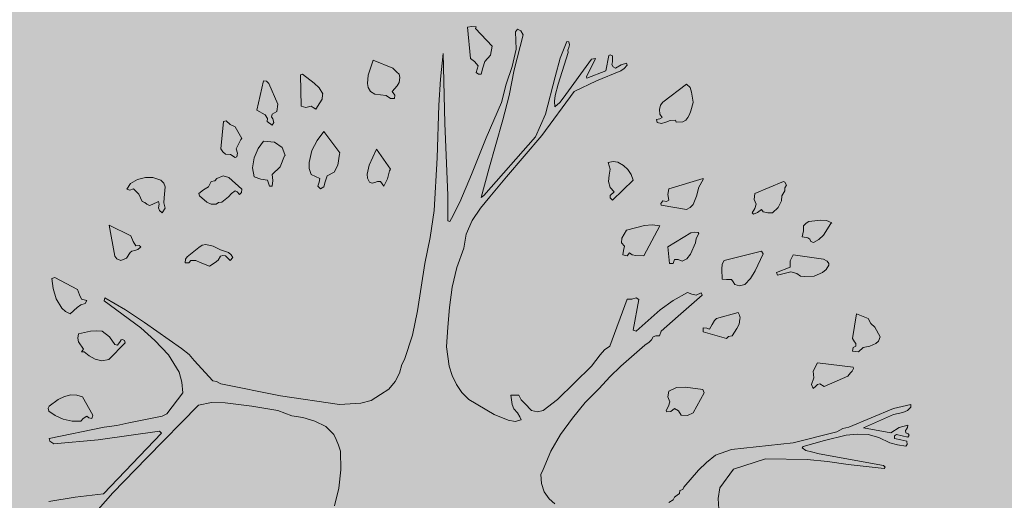
# Model space of a CAD drawing. Units: inches. Extents: x 84 to 1044, y -280 to 906.
# Tile 38 of 105: x 876 to 915, y -107 to -88. Entities that reach past the tile are written whole.
import ezdxf

# ---------------------------------------------------------------- set-up
doc = ezdxf.new("R2010")
doc.units = ezdxf.units.IN
doc.layers.add('L-PLNT', color=114, linetype='Continuous', lineweight=15)
doc.layers.add('L-PLNT-PATT', color=9, linetype='Continuous', lineweight=9, true_color=0xafd9aa)

# ---------------------------------------------------------------- blocks, each defined once
blk = doc.blocks.new('A$C37E508DF')
for p, q in [((0.6367, 1.5175), (0.6423, 1.5201)), ((0.6423, 1.5201), (0.6453, 1.5158)), ((0.6826, 1.493), (0.7096, 1.5209)), ((0.7083, 1.5239), (0.7152, 1.5244)), ((0.7096, 1.5209), (0.7083, 1.5239)), ((0.7152, 1.5244), (0.7225, 1.5231)), ((0.7225, 1.5231), (0.7174, 1.4729)), ((0.6329, 1.5111), (0.6367, 1.5175)), ((0.6475, 1.4545), (0.6329, 1.5111)), ((0.6453, 1.5158), (0.644, 1.4879)), ((0.5583, 1.4948), (0.5596, 1.4995)), ((0.5596, 1.4905), (0.5583, 1.4948)), ((0.5596, 1.4995), (0.563, 1.5003)), ((0.5613, 1.4862), (0.5596, 1.4905)), ((0.5608, 1.4823), (0.5613, 1.4862)), ((0.563, 1.5003), (0.5737, 1.4733)), ((0.644, 1.4879), (0.6505, 1.46)), ((0.6852, 1.4785), (0.6826, 1.493)), ((0.4897, 1.4772), (0.4935, 1.4789)), ((0.4897, 1.4678), (0.4897, 1.4772)), ((0.4935, 1.4789), (0.4952, 1.478)), ((0.4952, 1.478), (0.5004, 1.4532)), ((0.5313, 1.4437), (0.5167, 1.4729)), ((0.5167, 1.4729), (0.5231, 1.4716)), ((0.5231, 1.4716), (0.5686, 1.409)), ((0.5767, 1.4317), (0.5608, 1.4823)), ((0.5737, 1.4733), (0.5814, 1.4437)), ((0.6946, 1.4682), (0.6852, 1.4785)), ((0.7174, 1.4729), (0.7109, 1.4682)), ((0.7589, 1.3691), (0.7615, 1.481)), ((0.7615, 1.481), (0.7658, 1.4395)), ((0.8421, 1.4575), (0.8739, 1.4703)), ((0.8739, 1.4703), (0.882, 1.4463)), ((0.4657, 1.4622), (0.4669, 1.4652)), ((0.4708, 1.4566), (0.4657, 1.4622)), ((0.4669, 1.4652), (0.4755, 1.463)), ((0.4764, 1.4532), (0.4708, 1.4566)), ((0.4755, 1.463), (0.4845, 1.4575)), ((0.4845, 1.4575), (0.4884, 1.4596)), ((0.4884, 1.4596), (0.4905, 1.4635)), ((0.4905, 1.4635), (0.4897, 1.4678)), ((0.6552, 1.4137), (0.6475, 1.4545)), ((0.6505, 1.46), (0.6603, 1.4317)), ((0.6976, 1.4579), (0.6946, 1.4682)), ((0.7002, 1.4476), (0.6976, 1.4579)), ((0.7109, 1.4682), (0.7053, 1.4609)), ((0.7053, 1.4609), (0.7083, 1.4502)), ((0.8357, 1.451), (0.8421, 1.4575)), ((0.5154, 1.4373), (0.4764, 1.4532)), ((0.5004, 1.4532), (0.5308, 1.4412)), ((0.5308, 1.4412), (0.5313, 1.4437)), ((0.5814, 1.4437), (0.5969, 1.3833)), ((0.7049, 1.448), (0.7002, 1.4476)), ((0.7083, 1.4502), (0.7049, 1.448)), ((0.7658, 1.4395), (0.7684, 1.3979)), ((0.831, 1.4424), (0.8323, 1.4476)), ((0.8318, 1.4343), (0.831, 1.4424)), ((0.8323, 1.4476), (0.8357, 1.451)), ((0.882, 1.4463), (0.8829, 1.433)), ((0.9686, 1.4334), (0.9875, 1.4476)), ((0.9875, 1.4476), (0.9905, 1.4467)), ((0.9905, 1.4467), (0.9896, 1.3966)), ((0.3628, 1.4189), (0.3649, 1.4266)), ((0.3649, 1.4266), (0.3709, 1.4317)), ((0.3709, 1.4317), (0.4086, 1.403)), ((0.551, 1.4197), (0.5154, 1.4373)), ((0.5814, 1.4133), (0.5767, 1.4317)), ((0.6603, 1.4317), (0.668, 1.4021)), ((0.8353, 1.4292), (0.8318, 1.4343)), ((0.8434, 1.4197), (0.8353, 1.4292)), ((0.8816, 1.4262), (0.8781, 1.4197)), ((0.8829, 1.433), (0.8816, 1.4262)), ((0.9545, 1.4159), (0.9605, 1.4257)), ((0.9605, 1.4257), (0.9686, 1.4334)), ((1.0269, 1.3996), (1.0411, 1.433)), ((1.0411, 1.433), (1.045, 1.4365)), ((1.045, 1.4365), (1.0497, 1.4369)), ((1.0497, 1.4369), (1.0604, 1.3901)), ((0.3598, 1.403), (0.3628, 1.4189)), ((0.6029, 1.3494), (0.551, 1.4197)), ((0.5686, 1.409), (0.5741, 1.4021)), ((0.5827, 1.4043), (0.5814, 1.4133)), ((0.6655, 1.3743), (0.6552, 1.4137)), ((0.8391, 1.4141), (0.8434, 1.4197)), ((0.8395, 1.4086), (0.8391, 1.4141)), ((0.846, 1.4086), (0.8395, 1.4086)), ((0.8528, 1.4137), (0.846, 1.4086)), ((0.8619, 1.4146), (0.8528, 1.4137)), ((0.8709, 1.4154), (0.8619, 1.4146)), ((0.8781, 1.4197), (0.8709, 1.4154)), ((0.9549, 1.4146), (0.9545, 1.4159)), ((0.9558, 1.4077), (0.9549, 1.4146)), ((0.9592, 1.4017), (0.9558, 1.4077)), ((0.3602, 1.4021), (0.3598, 1.403)), ((0.364, 1.3888), (0.3602, 1.4021)), ((0.4086, 1.403), (0.4125, 1.3979)), ((0.4125, 1.3979), (0.4142, 1.391)), ((0.5741, 1.4021), (0.5823, 1.3953)), ((0.5823, 1.3953), (0.5827, 1.4043)), ((0.668, 1.4021), (0.6925, 1.3455)), ((0.7684, 1.3979), (0.771, 1.3134)), ((0.966, 1.3914), (0.9592, 1.4017)), ((0.9703, 1.3944), (0.966, 1.3914)), ((0.9733, 1.3966), (0.9703, 1.3944)), ((0.9819, 1.3944), (0.9733, 1.3966)), ((0.9896, 1.3966), (0.9819, 1.3944)), ((1.0282, 1.3876), (1.0269, 1.3996)), ((0.3657, 1.3828), (0.364, 1.3888)), ((0.3683, 1.3781), (0.3657, 1.3828)), ((0.3718, 1.3738), (0.3683, 1.3781)), ((0.4134, 1.3837), (0.4099, 1.3781)), ((0.4099, 1.3781), (0.4134, 1.376)), ((0.4142, 1.391), (0.4134, 1.3837)), ((0.4134, 1.376), (0.4189, 1.3751)), ((0.5969, 1.3833), (0.6132, 1.3472)), ((1.0359, 1.3833), (1.0282, 1.3876)), ((1.0334, 1.37), (1.0351, 1.376)), ((1.0351, 1.376), (1.0368, 1.3794)), ((1.0368, 1.3794), (1.0359, 1.3833)), ((1.0471, 1.3824), (1.0432, 1.3764)), ((1.0432, 1.3764), (1.0441, 1.3717)), ((1.0604, 1.3901), (1.0471, 1.3824)), ((0.3765, 1.3713), (0.3718, 1.3738)), ((0.3872, 1.3708), (0.3765, 1.3713)), ((0.3885, 1.3738), (0.3872, 1.3708)), ((0.3971, 1.3734), (0.3885, 1.3738)), ((0.4039, 1.3704), (0.3971, 1.3734)), ((0.4108, 1.3683), (0.4039, 1.3704)), ((0.4176, 1.37), (0.4108, 1.3683)), ((0.4189, 1.3751), (0.4176, 1.37)), ((0.6882, 1.2949), (0.6655, 1.3743)), ((0.7538, 1.2529), (0.7589, 1.3691)), ((1.0359, 1.3661), (1.0334, 1.37)), ((1.0441, 1.3717), (1.0359, 1.3661)), ((1.0848, 1.3443), (1.0955, 1.3631)), ((1.0955, 1.3631), (1.1033, 1.367)), ((1.1033, 1.367), (1.1097, 1.373)), ((1.1097, 1.373), (1.114, 1.3717)), ((1.114, 1.3717), (1.1183, 1.328)), ((0.6595, 1.2829), (0.6029, 1.3494)), ((0.6132, 1.3472), (0.6959, 1.2529)), ((0.6925, 1.3455), (0.7161, 1.2868)), ((0.9274, 1.3215), (0.9532, 1.3554)), ((0.9532, 1.3554), (0.9635, 1.3413)), ((1.0861, 1.343), (1.0848, 1.3443)), ((0.9635, 1.3413), (0.9721, 1.325)), ((1.0171, 1.3232), (1.0197, 1.3297)), ((1.0197, 1.3297), (1.0321, 1.3387)), ((1.0321, 1.3387), (1.0497, 1.3404)), ((1.0497, 1.3404), (1.0587, 1.3284)), ((1.0587, 1.3284), (1.0651, 1.3134)), ((1.0938, 1.328), (1.0861, 1.343)), ((0.771, 1.3134), (0.7761, 1.2285)), ((0.846, 1.2949), (0.8687, 1.3271)), ((0.8687, 1.3271), (0.8803, 1.3014)), ((0.9279, 1.3194), (0.9274, 1.3215)), ((0.9305, 1.3018), (0.9279, 1.3194)), ((0.9721, 1.325), (0.9768, 1.3061)), ((1.0149, 1.3172), (1.0171, 1.3232)), ((1.0162, 1.3164), (1.0149, 1.3172)), ((1.0231, 1.2988), (1.0162, 1.3164)), ((1.0651, 1.3134), (1.0677, 1.2975)), ((1.0917, 1.3207), (1.0938, 1.328)), ((1.0925, 1.3151), (1.0917, 1.3207)), ((1.0955, 1.3138), (1.0925, 1.3151)), ((1.1028, 1.3185), (1.0955, 1.3138)), ((1.111, 1.3194), (1.1028, 1.3185)), ((1.1153, 1.3228), (1.111, 1.3194)), ((1.1183, 1.328), (1.1153, 1.3228)), ((0.4648, 1.2945), (0.4717, 1.3009)), ((0.4717, 1.3009), (0.4807, 1.3065)), ((0.4807, 1.3065), (0.4884, 1.3074)), ((0.4884, 1.3074), (0.4965, 1.3057)), ((0.4965, 1.3057), (0.4935, 1.2954)), ((0.8803, 1.3014), (0.8833, 1.2872)), ((0.9365, 1.2902), (0.9305, 1.3018)), ((0.9768, 1.3061), (0.9763, 1.2962)), ((1.0359, 1.2868), (1.0231, 1.2988)), ((1.0677, 1.2975), (1.0647, 1.2829)), ((0.4562, 1.2774), (0.4597, 1.2868)), ((0.4597, 1.2868), (0.4648, 1.2945)), ((0.4935, 1.2954), (0.4948, 1.2855)), ((0.4948, 1.2855), (0.4961, 1.2756)), ((0.6865, 1.2508), (0.6595, 1.2829)), ((0.7002, 1.2495), (0.6882, 1.2949)), ((0.7161, 1.2868), (0.7349, 1.2422)), ((0.8473, 1.2924), (0.846, 1.2949)), ((0.8507, 1.2795), (0.8473, 1.2924)), ((0.8829, 1.2808), (0.8799, 1.2744)), ((0.8833, 1.2872), (0.8829, 1.2808)), ((0.9476, 1.2842), (0.9365, 1.2902)), ((0.951, 1.2748), (0.9476, 1.2842)), ((0.9733, 1.2868), (0.9596, 1.2799)), ((0.9763, 1.2962), (0.9733, 1.2868)), ((1.0347, 1.2769), (1.0359, 1.2868)), ((1.0647, 1.2829), (1.0544, 1.2791)), ((1.0848, 1.2628), (1.1054, 1.2817)), ((1.1054, 1.2817), (1.1148, 1.2842)), ((1.1148, 1.2842), (1.1247, 1.2804)), ((1.2147, 1.2774), (1.2276, 1.2817)), ((1.2276, 1.2817), (1.2392, 1.2817)), ((1.2392, 1.2817), (1.2521, 1.2787)), ((0.2101, 1.2696), (0.2127, 1.2744)), ((0.2127, 1.2654), (0.2101, 1.2696)), ((0.2127, 1.2744), (0.2152, 1.2752)), ((0.2127, 1.2602), (0.2127, 1.2654)), ((0.2152, 1.2752), (0.2611, 1.2559)), ((0.3439, 1.2804), (0.3992, 1.2636)), ((0.3439, 1.2787), (0.3439, 1.2804)), ((0.3507, 1.2662), (0.3439, 1.2787)), ((0.3546, 1.2516), (0.3507, 1.2662)), ((0.4897, 1.2452), (0.4562, 1.2774)), ((0.4935, 1.2658), (0.4867, 1.2589)), ((0.4961, 1.2756), (0.4935, 1.2658)), ((0.8567, 1.2679), (0.8507, 1.2795)), ((0.8619, 1.2752), (0.8567, 1.2679)), ((0.867, 1.2752), (0.8619, 1.2752)), ((0.8713, 1.2739), (0.867, 1.2752)), ((0.8756, 1.2726), (0.8713, 1.2739)), ((0.8799, 1.2744), (0.8756, 1.2726)), ((0.9532, 1.2666), (0.951, 1.2748)), ((0.9583, 1.2636), (0.9532, 1.2666)), ((0.9626, 1.2679), (0.9583, 1.2636)), ((0.9596, 1.2799), (0.9605, 1.2744)), ((0.9605, 1.2744), (0.9626, 1.2679)), ((1.0359, 1.2679), (1.0347, 1.2769)), ((1.0402, 1.2679), (1.0359, 1.2679)), ((1.0432, 1.2774), (1.0402, 1.2679)), ((1.0544, 1.2791), (1.0432, 1.2774)), ((1.1247, 1.2804), (1.1281, 1.2765)), ((1.1281, 1.2765), (1.1341, 1.2752)), ((1.1341, 1.2752), (1.1384, 1.2666)), ((1.1384, 1.2666), (1.1461, 1.2619)), ((1.2075, 1.2666), (1.21, 1.2726)), ((1.2096, 1.2491), (1.2075, 1.2666)), ((1.21, 1.2726), (1.2147, 1.2774)), ((1.2521, 1.2787), (1.2632, 1.2722)), ((1.2632, 1.2722), (1.2692, 1.2628)), ((0.2174, 1.2521), (0.2127, 1.2602)), ((0.2182, 1.2443), (0.2174, 1.2521)), ((0.2611, 1.2559), (0.262, 1.2465)), ((0.3602, 1.2383), (0.3546, 1.2516)), ((0.3992, 1.2636), (0.4005, 1.2546)), ((0.4005, 1.2546), (0.3992, 1.2452)), ((0.4867, 1.2589), (0.4935, 1.2529)), ((0.4931, 1.2491), (0.4897, 1.2452)), ((0.4935, 1.2529), (0.4931, 1.2491)), ((0.7015, 1.2323), (0.6865, 1.2508)), ((0.6959, 1.2529), (0.7002, 1.2495)), ((0.7538, 1.2122), (0.7538, 1.2529)), ((1.0852, 1.2576), (1.0848, 1.2628)), ((1.0883, 1.2546), (1.0852, 1.2576)), ((1.0921, 1.2585), (1.0883, 1.2546)), ((1.0955, 1.2602), (1.0921, 1.2585)), ((1.1015, 1.2559), (1.0955, 1.2602)), ((1.1063, 1.2508), (1.1015, 1.2559)), ((1.117, 1.2422), (1.1063, 1.2508)), ((1.1526, 1.2521), (1.141, 1.2422)), ((1.1461, 1.2619), (1.1539, 1.2559)), ((1.1539, 1.2559), (1.1526, 1.2521)), ((1.21, 1.2409), (1.2096, 1.2491)), ((1.2503, 1.2551), (1.2448, 1.2431)), ((1.2585, 1.2636), (1.2503, 1.2551)), ((1.2645, 1.2615), (1.2585, 1.2636)), ((1.2692, 1.2628), (1.2645, 1.2615)), ((0.2234, 1.2336), (0.2182, 1.2443)), ((0.2328, 1.2251), (0.2234, 1.2336)), ((0.262, 1.2465), (0.2586, 1.2388)), ((0.2586, 1.2388), (0.2611, 1.2319)), ((0.3649, 1.2336), (0.3602, 1.2383)), ((0.3709, 1.2306), (0.3649, 1.2336)), ((0.4112, 1.2375), (0.3709, 1.2306)), ((0.3992, 1.2452), (0.4026, 1.2431)), ((0.4026, 1.2431), (0.4086, 1.2443)), ((0.4086, 1.2443), (0.4121, 1.2401)), ((0.4121, 1.2401), (0.4112, 1.2375)), ((0.7349, 1.2422), (0.7482, 1.216)), ((1.1221, 1.2418), (1.117, 1.2422)), ((1.126, 1.2388), (1.1221, 1.2418)), ((1.1337, 1.2388), (1.126, 1.2388)), ((1.141, 1.2422), (1.1337, 1.2388)), ((1.2079, 1.2323), (1.21, 1.2409)), ((1.2186, 1.2332), (1.2169, 1.2285)), ((1.2186, 1.2431), (1.2173, 1.2392)), ((1.2173, 1.2392), (1.2186, 1.2332)), ((1.2285, 1.2383), (1.2186, 1.2431)), ((1.2328, 1.2366), (1.2285, 1.2383)), ((1.2371, 1.2388), (1.2328, 1.2366)), ((1.2405, 1.2418), (1.2371, 1.2388)), ((1.2448, 1.2431), (1.2405, 1.2418)), ((0.2401, 1.2251), (0.2328, 1.2251)), ((0.2474, 1.2268), (0.2401, 1.2251)), ((0.2504, 1.2306), (0.2474, 1.2268)), ((0.2568, 1.2255), (0.2504, 1.2306)), ((0.2633, 1.2229), (0.2568, 1.2255)), ((0.2611, 1.2319), (0.265, 1.2251)), ((0.265, 1.2251), (0.2633, 1.2229)), ((0.7148, 1.2126), (0.7015, 1.2323)), ((0.7761, 1.2285), (0.7821, 1.1856)), ((1.2126, 1.2251), (1.2079, 1.2323)), ((1.2169, 1.2285), (1.2126, 1.2251)), ((0.1376, 1.2092), (0.1458, 1.2126)), ((0.1389, 1.2079), (0.1376, 1.2092)), ((0.1505, 1.189), (0.1389, 1.2079)), ((0.1458, 1.2126), (0.1548, 1.2135)), ((0.1548, 1.2135), (0.1741, 1.2109)), ((0.1741, 1.2109), (0.1784, 1.2083)), ((0.1784, 1.2083), (0.1831, 1.204)), ((0.1831, 1.204), (0.1831, 1.1959)), ((0.4134, 1.204), (0.4258, 1.2058)), ((0.4391, 1.156), (0.4134, 1.204)), ((0.4258, 1.2058), (0.4382, 1.2045)), ((0.4382, 1.2045), (0.4669, 1.1972)), ((0.7246, 1.1908), (0.7148, 1.2126)), ((0.7482, 1.216), (0.7508, 1.2109)), ((0.7508, 1.2109), (0.7538, 1.2122)), ((1.2628, 1.1882), (1.2975, 1.2053)), ((1.2975, 1.2053), (1.2885, 1.1556)), ((0.1582, 1.1822), (0.1505, 1.189)), ((0.1848, 1.1865), (0.1788, 1.1852)), ((0.1831, 1.1959), (0.1848, 1.1865)), ((0.3507, 1.1916), (0.352, 1.1933)), ((0.355, 1.1839), (0.3507, 1.1916)), ((0.352, 1.1933), (0.3576, 1.1942)), ((0.3576, 1.1942), (0.364, 1.1929)), ((0.364, 1.1929), (0.4005, 1.1702)), ((0.4669, 1.1972), (0.4747, 1.1843)), ((0.7281, 1.168), (0.7246, 1.1908)), ((1.2589, 1.1792), (1.2628, 1.1882)), ((0.1668, 1.1775), (0.1582, 1.1822)), ((0.1711, 1.1792), (0.1668, 1.1775)), ((0.1728, 1.1826), (0.1711, 1.1792)), ((0.1758, 1.1847), (0.1728, 1.1826)), ((0.1788, 1.1852), (0.1758, 1.1847)), ((0.3563, 1.177), (0.355, 1.1839)), ((0.3645, 1.1586), (0.3563, 1.177)), ((0.4005, 1.1702), (0.3979, 1.1436)), ((0.4751, 1.177), (0.47, 1.1714)), ((0.47, 1.1714), (0.4721, 1.1646)), ((0.4747, 1.1843), (0.4751, 1.177)), ((0.7821, 1.1856), (0.7911, 1.1436)), ((1.1187, 1.1655), (1.1307, 1.1714)), ((1.1307, 1.1714), (1.1423, 1.1744)), ((1.1423, 1.1744), (1.1483, 1.1732)), ((1.1483, 1.1732), (1.1539, 1.1693)), ((1.2469, 1.1702), (1.2495, 1.1723)), ((1.2478, 1.1693), (1.2469, 1.1702)), ((1.2495, 1.1723), (1.2546, 1.1719)), ((1.2546, 1.1719), (1.2589, 1.1792)), ((0.1509, 1.1504), (0.1994, 1.1573)), ((0.1994, 1.1573), (0.2041, 1.1479)), ((0.2478, 1.1594), (0.2504, 1.1637)), ((0.2607, 1.1316), (0.2478, 1.1594)), ((0.2504, 1.1637), (0.3104, 1.1487)), ((0.37, 1.1509), (0.3645, 1.1586)), ((0.4519, 1.1564), (0.4391, 1.156)), ((0.458, 1.1573), (0.4519, 1.1564)), ((0.4622, 1.1607), (0.458, 1.1573)), ((0.4657, 1.156), (0.4622, 1.1607)), ((0.473, 1.1573), (0.4657, 1.156)), ((0.4721, 1.1646), (0.473, 1.1573)), ((0.7396, 1.1371), (0.7281, 1.168)), ((1.099, 1.153), (1.102, 1.1573)), ((1.102, 1.1573), (1.1063, 1.1612)), ((1.111, 1.156), (1.1033, 1.1487)), ((1.1063, 1.1612), (1.1187, 1.1655)), ((1.1153, 1.1564), (1.111, 1.156)), ((1.1191, 1.1556), (1.1153, 1.1564)), ((1.1226, 1.1492), (1.1191, 1.1556)), ((1.1539, 1.1693), (1.1727, 1.1543)), ((1.1727, 1.1543), (1.1749, 1.1504)), ((1.2516, 1.1659), (1.2478, 1.1693)), ((1.2563, 1.1646), (1.2516, 1.1659)), ((1.2611, 1.1637), (1.2563, 1.1646)), ((1.2641, 1.1612), (1.2611, 1.1637)), ((1.2701, 1.1522), (1.2641, 1.1612)), ((1.2885, 1.1556), (1.2851, 1.1509)), ((0.1419, 1.1436), (0.1449, 1.1474)), ((0.1419, 1.141), (0.1419, 1.1436)), ((0.1462, 1.1342), (0.1419, 1.141)), ((0.1449, 1.1474), (0.1509, 1.1504)), ((0.2041, 1.1479), (0.2045, 1.138)), ((0.3104, 1.1487), (0.3134, 1.1423)), ((0.3134, 1.1423), (0.3139, 1.1346)), ((0.3778, 1.1474), (0.37, 1.1509)), ((0.3842, 1.15), (0.3778, 1.1474)), ((0.3898, 1.15), (0.3842, 1.15)), ((0.3923, 1.1436), (0.3898, 1.15)), ((0.3979, 1.1436), (0.3923, 1.1436)), ((0.7911, 1.1436), (0.8027, 1.0677)), ((1.1033, 1.1487), (1.099, 1.153)), ((1.1273, 1.1453), (1.1226, 1.1492)), ((1.1367, 1.1393), (1.1273, 1.1453)), ((1.1517, 1.1453), (1.1367, 1.1393)), ((1.1586, 1.1483), (1.1517, 1.1453)), ((1.1663, 1.1487), (1.1586, 1.1483)), ((1.1697, 1.1449), (1.1663, 1.1487)), ((1.1757, 1.1449), (1.1697, 1.1449)), ((1.1749, 1.1504), (1.1757, 1.1449)), ((1.2791, 1.1487), (1.2701, 1.1522)), ((1.2851, 1.1509), (1.2791, 1.1487)), ((0.1522, 1.1294), (0.1462, 1.1342)), ((0.1655, 1.1234), (0.1522, 1.1294)), ((0.181, 1.1226), (0.1655, 1.1234)), ((0.1878, 1.1234), (0.181, 1.1226)), ((0.1938, 1.1273), (0.1878, 1.1234)), ((0.2032, 1.1303), (0.1938, 1.1273)), ((0.2247, 1.1251), (0.2032, 1.1303)), ((0.2045, 1.138), (0.226, 1.129)), ((0.226, 1.129), (0.2247, 1.1251)), ((0.268, 1.1196), (0.2607, 1.1316)), ((0.3139, 1.1346), (0.3134, 1.1183)), ((0.7469, 1.1054), (0.7396, 1.1371)), ((0.277, 1.1101), (0.268, 1.1196)), ((0.2856, 1.108), (0.277, 1.1101)), ((0.2933, 1.1101), (0.2856, 1.108)), ((0.2959, 1.1144), (0.2933, 1.1101)), ((0.2984, 1.1179), (0.2959, 1.1144)), ((0.3066, 1.1179), (0.2984, 1.1179)), ((0.3134, 1.1183), (0.3066, 1.1179)), ((1.3485, 1.102), (1.385, 1.1209)), ((1.385, 1.1209), (1.3897, 1.1196)), ((1.3897, 1.1196), (1.3875, 1.1037)), ((0.3456, 1.093), (0.3469, 1.0964)), ((0.3842, 1.0591), (0.3456, 1.093)), ((0.3469, 1.0964), (0.355, 1.093)), ((0.355, 1.093), (0.3619, 1.0943)), ((0.3619, 1.0943), (0.3692, 1.0968)), ((0.3692, 1.0968), (0.3923, 1.0844)), ((0.7512, 1.0728), (0.7469, 1.1054)), ((1.3421, 1.0861), (1.3455, 1.0934)), ((1.3455, 1.0934), (1.3485, 1.102)), ((1.3875, 1.1037), (1.3828, 1.087)), ((0.3923, 1.0844), (0.4129, 1.069)), ((0.4472, 1.0857), (0.4515, 1.0887)), ((0.4562, 1.0364), (0.4472, 1.0857)), ((0.4515, 1.0887), (0.4584, 1.0865)), ((0.4584, 1.0865), (0.4657, 1.0861)), ((0.4657, 1.0861), (0.4939, 1.0107)), ((1.3057, 1.0835), (1.2469, 1.0402)), ((1.2713, 1.0694), (1.3044, 1.0887)), ((1.3044, 1.0887), (1.3057, 1.0835)), ((1.3335, 1.0844), (1.3421, 1.0861)), ((1.3361, 1.0793), (1.3335, 1.0844)), ((1.3434, 1.0771), (1.3361, 1.0793)), ((1.349, 1.0728), (1.3434, 1.0771)), ((1.3828, 1.087), (1.3738, 1.072)), ((0.0789, 1.0552), (0.0978, 1.063)), ((0.0978, 1.063), (0.1042, 1.0231)), ((0.2847, 1.0565), (0.2856, 1.0604)), ((0.2856, 1.0604), (0.2877, 1.0647)), ((0.2877, 1.0647), (0.3224, 1.0552)), ((0.4129, 1.069), (0.4515, 1.0351)), ((0.7538, 1.0415), (0.7512, 1.0728)), ((0.8027, 1.0677), (0.8108, 1.0287)), ((1.2409, 1.0488), (1.2713, 1.0694)), ((1.3605, 1.063), (1.349, 1.0728)), ((1.3678, 1.0664), (1.3605, 1.063)), ((1.3738, 1.072), (1.3678, 1.0664)), ((0.0682, 1.0415), (0.0746, 1.0475)), ((0.0746, 1.0475), (0.0789, 1.0552)), ((0.2851, 1.054), (0.2847, 1.0565)), ((0.2864, 1.0463), (0.2851, 1.054)), ((0.2899, 1.039), (0.2864, 1.0463)), ((0.3224, 1.0552), (0.3255, 1.0522)), ((0.3255, 1.0522), (0.3293, 1.0458)), ((0.3293, 1.0458), (0.3336, 1.0381)), ((0.4112, 1.0351), (0.3842, 1.0591)), ((1.1813, 1.0072), (1.2409, 1.0488)), ((0.0596, 1.0257), (0.0682, 1.0415)), ((0.2972, 1.0274), (0.2899, 1.039)), ((0.3439, 1.0338), (0.3066, 1.0231)), ((0.3336, 1.0381), (0.3383, 1.0398)), ((0.3383, 1.0398), (0.3439, 1.0402)), ((0.3439, 1.0402), (0.3439, 1.0338)), ((0.4138, 1.0274), (0.4112, 1.0351)), ((0.4515, 1.0351), (0.4562, 1.0364)), ((0.7559, 1.0098), (0.7538, 1.0415)), ((0.8108, 1.0287), (0.8233, 0.9892)), ((1.2469, 1.0402), (1.2246, 1.0201)), ((1.2971, 1.0257), (1.3091, 1.0351)), ((1.3091, 1.0351), (1.3185, 1.0355)), ((1.3185, 1.0355), (1.3275, 1.0347)), ((1.3275, 1.0347), (1.3468, 1.0308)), ((1.3468, 1.0308), (1.3481, 1.0239)), ((0.0626, 1.0188), (0.0596, 1.0257)), ((0.0665, 1.0149), (0.0626, 1.0188)), ((0.0763, 1.0111), (0.0665, 1.0149)), ((0.1012, 1.018), (0.099, 1.0149)), ((0.099, 1.0149), (0.099, 1.0111)), ((0.1042, 1.0231), (0.1012, 1.018)), ((0.3032, 1.0265), (0.2972, 1.0274)), ((0.3066, 1.0231), (0.3032, 1.0265)), ((0.4202, 1.0274), (0.4138, 1.0274)), ((0.4241, 1.0257), (0.4202, 1.0274)), ((0.4267, 1.0209), (0.4241, 1.0257)), ((0.4305, 1.0175), (0.4267, 1.0209)), ((0.4378, 1.0124), (0.4305, 1.0175)), ((0.476, 0.9789), (0.4378, 1.0124)), ((1.2246, 1.0201), (1.2023, 0.9969)), ((1.2718, 1.0162), (1.2731, 1.0197)), ((1.2984, 0.9892), (1.2718, 1.0162)), ((1.2731, 1.0197), (1.2761, 1.0218)), ((1.2761, 1.0218), (1.2786, 1.0209)), ((1.2786, 1.0209), (1.2799, 1.0184)), ((1.2799, 1.0184), (1.2842, 1.0124)), ((1.2842, 1.0124), (1.2885, 1.0136)), ((1.2885, 1.0136), (1.2971, 1.0257)), ((1.3468, 1.018), (1.3391, 1.0059)), ((1.3481, 1.0239), (1.3468, 1.018)), ((0.087, 1.0085), (0.0763, 1.0111)), ((0.0948, 1.0016), (0.087, 1.0085)), ((0.1042, 1.0029), (0.0948, 1.0016)), ((0.099, 1.0111), (0.1033, 1.0085)), ((0.1033, 1.0085), (0.1042, 1.0029)), ((0.4939, 1.0107), (0.5021, 1.0051)), ((0.5021, 1.0051), (0.5094, 0.9969)), ((0.5094, 0.9969), (0.5231, 0.9789)), ((0.7516, 0.9785), (0.7559, 1.0098)), ((1.1612, 0.9879), (1.1693, 0.9974)), ((1.1693, 0.9974), (1.1813, 1.0072)), ((1.2023, 0.9969), (1.1852, 0.9691)), ((1.3378, 1.0016), (1.3297, 0.9952)), ((1.3421, 1.0016), (1.3378, 1.0016)), ((1.3391, 1.0059), (1.3421, 1.0016)), ((0.1029, 0.9772), (0.1604, 0.9841)), ((0.1604, 0.9841), (0.1672, 0.9708)), ((0.8233, 0.9892), (0.8275, 0.9815)), ((0.8275, 0.9815), (0.8314, 0.9673)), ((1.1311, 0.9549), (1.1612, 0.9879)), ((1.3095, 0.9875), (1.2984, 0.9892)), ((1.3202, 0.9901), (1.3095, 0.9875)), ((1.3297, 0.9952), (1.3202, 0.9901)), ((0.1025, 0.9751), (0.1029, 0.9772)), ((0.1046, 0.9708), (0.1025, 0.9751)), ((0.1076, 0.9682), (0.1046, 0.9708)), ((0.1119, 0.9626), (0.1076, 0.9682)), ((0.1672, 0.9708), (0.1664, 0.9601)), ((0.4939, 0.9618), (0.476, 0.9789)), ((0.5231, 0.9789), (0.578, 0.9253)), ((0.7469, 0.9635), (0.7516, 0.9785)), ((0.8314, 0.9673), (0.8383, 0.954)), ((1.1852, 0.9691), (1.1809, 0.9532)), ((0.1496, 0.9463), (0.1119, 0.9626)), ((0.1565, 0.9506), (0.1496, 0.9463)), ((0.1604, 0.9493), (0.1565, 0.9506)), ((0.1629, 0.9468), (0.1604, 0.9493)), ((0.1664, 0.9601), (0.1698, 0.9493)), ((0.1698, 0.9493), (0.1672, 0.9429)), ((0.5111, 0.9429), (0.4939, 0.9618)), ((0.7315, 0.9365), (0.7401, 0.9493)), ((0.7401, 0.9493), (0.7469, 0.9635)), ((0.8383, 0.954), (0.8486, 0.942)), ((1.0227, 0.9309), (1.1183, 0.9506)), ((1.1183, 0.9506), (1.1256, 0.954)), ((1.1256, 0.954), (1.1311, 0.9549)), ((1.1809, 0.9532), (1.1796, 0.936)), ((0.1672, 0.9429), (0.1629, 0.9468)), ((0.3426, 0.936), (0.3443, 0.9412)), ((0.3602, 0.9039), (0.3426, 0.936)), ((0.3443, 0.9412), (0.3722, 0.9451)), ((0.3722, 0.9451), (0.3868, 0.9446)), ((0.3868, 0.9446), (0.3992, 0.9386)), ((0.3992, 0.9386), (0.4009, 0.9292)), ((0.5334, 0.9202), (0.5111, 0.9429)), ((0.7203, 0.9253), (0.7315, 0.9365)), ((0.8486, 0.942), (0.8619, 0.933)), ((0.8619, 0.933), (0.8769, 0.9236)), ((1.1796, 0.936), (1.2049, 0.9022)), ((0.0103, 0.9129), (0.0103, 0.9172)), ((0.0103, 0.9172), (0.0382, 0.9107)), ((0.4009, 0.9292), (0.3975, 0.9215)), ((0.3975, 0.9215), (0.3996, 0.9142)), ((0.554, 0.8953), (0.5334, 0.9202)), ((0.578, 0.9253), (0.6011, 0.9077)), ((0.6196, 0.9077), (0.6303, 0.9189)), ((0.6303, 0.9189), (0.6359, 0.9245)), ((0.6359, 0.9245), (0.6397, 0.9322)), ((0.6397, 0.9322), (0.653, 0.9322)), ((0.6505, 0.9172), (0.6479, 0.9103)), ((0.653, 0.9322), (0.6505, 0.9172)), ((0.6796, 0.9013), (0.7203, 0.9253)), ((0.8769, 0.9236), (0.8936, 0.9193)), ((0.8936, 0.9193), (0.9279, 0.9172)), ((0.9279, 0.9172), (1.0227, 0.9309)), ((1.1114, 0.9198), (1.0685, 0.9142)), ((1.1333, 0.9202), (1.1114, 0.9198)), ((1.1543, 0.9159), (1.1333, 0.9202)), ((1.3241, 0.9), (1.3404, 0.9292)), ((1.3404, 0.9292), (1.3494, 0.9322)), ((1.3494, 0.9322), (1.3592, 0.9326)), ((1.3592, 0.9326), (1.3695, 0.93)), ((1.3695, 0.93), (1.3794, 0.9253)), ((1.3794, 0.9253), (1.394, 0.9146)), ((0.0159, 0.9073), (0.0103, 0.9129)), ((0.0232, 0.9043), (0.0159, 0.9073)), ((0.0386, 0.9013), (0.0232, 0.9043)), ((0.0382, 0.9107), (0.1098, 0.8807)), ((0.0866, 0.8794), (0.0386, 0.9013)), ((0.3692, 0.8992), (0.3602, 0.9039)), ((0.3838, 0.9069), (0.379, 0.9)), ((0.3898, 0.9107), (0.3838, 0.9069)), ((0.3958, 0.906), (0.3898, 0.9107)), ((0.4026, 0.9052), (0.3958, 0.906)), ((0.3996, 0.9142), (0.4031, 0.9077)), ((0.4031, 0.9077), (0.4026, 0.9052)), ((0.6011, 0.9077), (0.6097, 0.9056)), ((0.6097, 0.9056), (0.6196, 0.9077)), ((0.6423, 0.9039), (0.6384, 0.8974)), ((0.6479, 0.9103), (0.6423, 0.9039)), ((0.6569, 0.8919), (0.6796, 0.9013)), ((1.0269, 0.9077), (1.0042, 0.8987)), ((1.0685, 0.9142), (1.0269, 0.9077)), ((1.2371, 0.8314), (1.1543, 0.9159)), ((1.2049, 0.9022), (1.2126, 0.8983)), ((1.3948, 0.9065), (1.3846, 0.8992)), ((1.394, 0.9146), (1.3957, 0.9112)), ((1.3957, 0.9112), (1.3948, 0.9065)), ((0.379, 0.9), (0.3692, 0.8992)), ((0.5728, 0.8691), (0.554, 0.8953)), ((0.6384, 0.8974), (0.6359, 0.8927)), ((0.6359, 0.8927), (0.6457, 0.8897)), ((0.6457, 0.8897), (0.6569, 0.8919)), ((0.9673, 0.8906), (0.9498, 0.8816)), ((0.9866, 0.8962), (0.9673, 0.8906)), ((1.0042, 0.8987), (0.9866, 0.8962)), ((1.2126, 0.8983), (1.2662, 0.8876)), ((1.2662, 0.8876), (1.2855, 0.8833)), ((1.3254, 0.8944), (1.3241, 0.9)), ((1.3301, 0.8957), (1.3254, 0.8944)), ((1.3335, 0.8983), (1.3301, 0.8957)), ((1.3395, 0.8944), (1.3335, 0.8983)), ((1.3434, 0.8906), (1.3395, 0.8944)), ((1.3571, 0.8906), (1.3434, 0.8906)), ((1.3713, 0.8936), (1.3571, 0.8906)), ((1.3846, 0.8992), (1.3713, 0.8936)), ((0.0133, 0.8679), (0.015, 0.87)), ((0.015, 0.87), (0.0184, 0.8717)), ((0.0159, 0.8803), (0.0154, 0.8837)), ((0.0154, 0.8837), (0.0292, 0.8803)), ((0.0176, 0.8777), (0.0159, 0.8803)), ((0.0193, 0.8752), (0.0176, 0.8777)), ((0.0184, 0.8717), (0.0193, 0.8752)), ((0.0292, 0.8803), (0.0424, 0.8717)), ((0.0424, 0.8717), (0.0866, 0.8794)), ((0.0965, 0.8696), (0.0789, 0.8687)), ((0.1141, 0.8679), (0.0965, 0.8696)), ((0.1098, 0.8807), (0.1196, 0.8786)), ((0.1196, 0.8786), (0.1295, 0.873)), ((0.1295, 0.873), (0.1994, 0.8554)), ((0.9498, 0.8816), (0.9369, 0.8687)), ((1.2169, 0.8743), (1.2135, 0.8713)), ((1.2135, 0.8713), (1.2491, 0.834)), ((1.3151, 0.8606), (1.2169, 0.8743)), ((1.2855, 0.8833), (1.3057, 0.8807)), ((1.3057, 0.8807), (1.394, 0.8623)), ((0.0154, 0.8649), (0.0133, 0.8679)), ((0.0334, 0.8687), (0.0154, 0.8649)), ((0.0163, 0.8529), (0.0171, 0.8584)), ((0.0171, 0.8584), (0.0266, 0.8602)), ((0.0266, 0.8602), (0.0369, 0.8623)), ((0.0442, 0.8554), (0.0317, 0.8524)), ((0.0369, 0.8666), (0.0334, 0.8687)), ((0.0369, 0.8623), (0.0369, 0.8666)), ((0.0617, 0.864), (0.0442, 0.8554)), ((0.0789, 0.8687), (0.0617, 0.864)), ((0.1492, 0.8593), (0.1141, 0.8679)), ((0.1835, 0.8499), (0.1492, 0.8593)), ((0.1994, 0.8554), (0.2984, 0.8447)), ((0.5887, 0.8421), (0.5728, 0.8691)), ((0.933, 0.861), (0.9296, 0.852)), ((0.9369, 0.8687), (0.933, 0.861)), ((1.3863, 0.8541), (1.3151, 0.8606)), ((1.3927, 0.8584), (1.3863, 0.8541)), ((1.394, 0.8623), (1.3927, 0.8584)), ((0.0184, 0.8503), (0.0163, 0.8529)), ((0.0317, 0.8524), (0.0184, 0.8503)), ((0.1578, 0.8378), (0.1698, 0.8413)), ((0.1698, 0.8413), (0.1792, 0.8434)), ((0.1792, 0.8434), (0.1848, 0.8477)), ((0.1848, 0.8477), (0.1835, 0.8499)), ((0.2984, 0.8447), (0.3242, 0.8357)), ((0.6007, 0.8125), (0.5887, 0.8421)), ((0.9262, 0.8421), (0.9257, 0.8121)), ((0.9296, 0.852), (0.9262, 0.8421)), ((0.0545, 0.8194), (0.1578, 0.8378)), ((0.1441, 0.8258), (0.1111, 0.8207)), ((0.1771, 0.8288), (0.1441, 0.8258)), ((0.2436, 0.8301), (0.1771, 0.8288)), ((0.2954, 0.813), (0.2436, 0.8301)), ((0.3242, 0.8357), (0.3387, 0.8241)), ((0.3387, 0.8241), (0.3512, 0.8117)), ((1.2919, 0.7752), (1.2371, 0.8314)), ((1.2491, 0.834), (1.3069, 0.7735)), ((0.0519, 0.8164), (0.0545, 0.8194)), ((0.0532, 0.8143), (0.0519, 0.8164)), ((0.1111, 0.8207), (0.0532, 0.8143)), ((0.3173, 0.7834), (0.2954, 0.813)), ((0.3512, 0.8117), (0.3748, 0.7842)), ((0.6046, 0.8048), (0.6007, 0.8125)), ((0.9257, 0.8121), (0.9287, 0.7825)), ((0.6037, 0.7903), (0.6046, 0.8048)), ((0.3199, 0.7662), (0.3173, 0.7834)), ((0.3748, 0.7842), (0.3765, 0.7804)), ((0.3765, 0.7804), (0.3816, 0.7791)), ((0.3816, 0.7791), (0.382, 0.7744)), ((0.5913, 0.7658), (0.599, 0.777)), ((0.599, 0.777), (0.6037, 0.7903)), ((0.9287, 0.7825), (0.936, 0.7542)), ((1.3151, 0.7487), (1.2919, 0.7752)), ((0.3186, 0.7491), (0.3199, 0.7662)), ((0.382, 0.7744), (0.3859, 0.7714)), ((0.3859, 0.7714), (0.3902, 0.7684)), ((0.3902, 0.7684), (0.3919, 0.7641)), ((0.3919, 0.7641), (0.3988, 0.7598)), ((0.5823, 0.7577), (0.5913, 0.7658)), ((1.3069, 0.7735), (1.352, 0.7684)), ((1.352, 0.7684), (1.3948, 0.7615))]:
    blk.add_line(p, q)

msp = doc.modelspace()

# ---------------------------------------------------------------- hatches: boundary and pattern name
at = {"layer": 'L-PLNT-PATT', "transparency": 33554597}
h = msp.add_hatch(color=256, dxfattribs=at)
h.dxf.hatch_style = 1
h.paths.add_polyline_path([(791.074, 31.12), (791.074, 91.12), (743.074, 91.12), (674.074, 91.12), (674.074, 31.12), (650.074, 31.12), (650.074, -112.88), (983.074, -112.88), (983.074, -64.88), (791.074, -64.88)])

# ---------------------------------------------------------------- block references
at = {"layer": 'L-PLNT', "xscale": -24.64361536662419, "yscale": 24.64361536662419, "zscale": 24.64361536662419}
msp.add_blockref('A$C37E508DF', (911.469, -125.52), dxfattribs=at)

doc.saveas('drawing.dxf')
